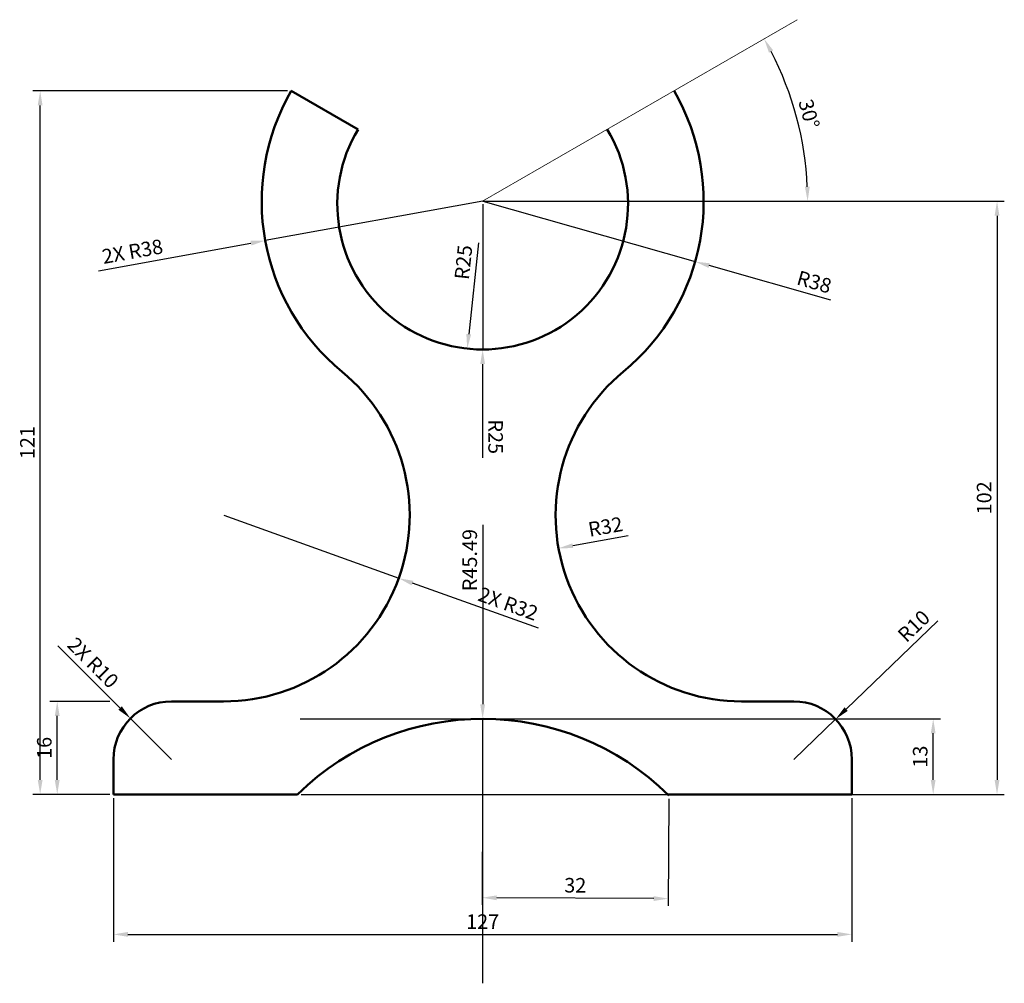
# Model space of a CAD drawing. Units: millimetres. Extents: x 195 to 364, y 6 to 172.
import ezdxf

# ---------------------------------------------------------------- set-up
doc = ezdxf.new("R2010")
doc.units = ezdxf.units.MM
for name, color, linetype, lineweight in [('M-CONS', 8, 'Continuous', 18), ('M-DIMS', 2, 'Continuous', 25), ('M-OUTL', 7, 'Continuous', 50)]:
    doc.layers.add(name, color=color, linetype=linetype, lineweight=lineweight)
doc.styles.get("Standard").update_dxf_attribs({"font": 'arial.ttf'})
doc.dimstyles.new('ISO-25', dxfattribs={"dimtxt": 2.5, "dimasz": 2.5, "dimexe": 1.25, "dimexo": 0.625, "dimtad": 1, "dimtxsty": 'Standard', "dimcen": 2.5, "dimadec": 0, "dimazin": 0, "dimtfac": 1, "dimtmove": 0, "dimatfit": 3, "dimfxl": 1, "dimarcsym": 0})

# ---------------------------------------------------------------- blocks, each defined once
blk = doc.blocks.new('*D1')
at = {"layer": 'Defpoints', "color": 0, "transparency": 16777216}
for p in [(328.48, 171.63), (329.42, 150.1), (274.38, 140.4), (274.38, 140.4), (329.43, 140.4)]:
    blk.add_point(p, dxfattribs=at)
at = {"layer": 'M-DIMS', "color": 0, "lineweight": -2, "transparency": 16777216}
blk.add_line((330.05, 140.4), (331.52, 140.4), dxfattribs=at)
blk.add_arc((274.38, 140.4), 55.89, 2.563, 27.437, dxfattribs=at)
at = {"layer": 'M-DIMS', "color": 0, "transparency": 16777216}
for points in [[(323.62, 165.95), (324.35, 166.35), (322.78, 168.34)], [(330.63, 142.91), (329.8, 142.89), (330.27, 140.4)]]:
    blk.add_solid(points, dxfattribs=at)
at = {"layer": 'M-DIMS', "color": 0, "transparency": 16777216, "insert": (330.2, 155.35), "char_height": 2.5, "attachment_point": 5, "rotation": 285}
blk.add_mtext('30°', dxfattribs=at)
blk = doc.blocks.new('*D2')
at = {"layer": 'Defpoints', "color": 0, "transparency": 16777216}
for p in [(274.38, 139.91), (271.72, 115.06)]:
    blk.add_point(p, dxfattribs=at)
at = {"layer": 'M-DIMS', "color": 0, "lineweight": -2, "transparency": 16777216}
blk.add_line((273.67, 133.27), (271.98, 117.54), dxfattribs=at)
at = {"layer": 'M-DIMS', "color": 0, "transparency": 16777216}
blk.add_solid([(271.57, 117.59), (272.4, 117.5), (271.72, 115.06)], dxfattribs=at)
at = {"layer": 'M-DIMS', "color": 0, "transparency": 16777216, "insert": (271.39, 129.87), "char_height": 2.5, "attachment_point": 5, "rotation": 83.8896}
blk.add_mtext('R25', dxfattribs=at)
blk = doc.blocks.new('*D3')
at = {"layer": 'Defpoints', "color": 0, "transparency": 16777216}
for p in [(318.92, 86.4), (287.43, 80.72)]:
    blk.add_point(p, dxfattribs=at)
at = {"layer": 'M-DIMS', "color": 0, "lineweight": -2, "transparency": 16777216}
blk.add_line((299.43, 82.89), (289.89, 81.17), dxfattribs=at)
at = {"layer": 'M-DIMS', "color": 0, "transparency": 16777216}
blk.add_solid([(289.81, 81.58), (289.96, 80.76), (287.43, 80.72)], dxfattribs=at)
at = {"layer": 'M-DIMS', "color": 0, "transparency": 16777216, "insert": (295.55, 84.12), "char_height": 2.5, "attachment_point": 5, "rotation": 10.2105}
blk.add_mtext('R32', dxfattribs=at)
blk = doc.blocks.new('*D4')
at = {"layer": 'Defpoints', "color": 0, "transparency": 16777216}
for p in [(335.08, 51.33), (327.88, 44.4)]:
    blk.add_point(p, dxfattribs=at)
at = {"layer": 'M-DIMS', "color": 0, "lineweight": -2, "transparency": 16777216}
for p, q in [((352.67, 68.25), (336.88, 53.06)), ((327.88, 44.4), (335.08, 51.33))]:
    blk.add_line(p, q, dxfattribs=at)
at = {"layer": 'M-DIMS', "color": 0, "transparency": 16777216}
blk.add_solid([(336.6, 53.36), (337.17, 52.76), (335.08, 51.33)], dxfattribs=at)
at = {"layer": 'M-DIMS', "color": 0, "transparency": 16777216, "insert": (348.75, 67.12), "char_height": 2.5, "attachment_point": 5, "rotation": 43.8985}
blk.add_mtext('R10', dxfattribs=at)
blk = doc.blocks.new('*D5')
at = {"layer": 'Defpoints', "color": 0, "transparency": 16777216}
for p in [(274.38, 38.4), (306.38, 38.24), (274.29, 20.63)]:
    blk.add_point(p, dxfattribs=at)
at = {"layer": 'M-DIMS', "color": 0, "lineweight": -2, "transparency": 16777216}
for p, q in [((274.37, 37.77), (274.28, 19.38)), ((306.37, 37.61), (306.28, 19.22)), ((303.79, 20.48), (276.79, 20.62))]:
    blk.add_line(p, q, dxfattribs=at)
at = {"layer": 'M-DIMS', "color": 0, "transparency": 16777216}
for points in [[(276.79, 21.03), (276.79, 20.2), (274.29, 20.63)], [(303.79, 20.9), (303.79, 20.07), (306.29, 20.47)]]:
    blk.add_solid(points, dxfattribs=at)
at = {"layer": 'M-DIMS', "color": 0, "transparency": 16777216, "insert": (290.3, 22.45), "char_height": 2.5, "attachment_point": 5, "rotation": 359.7141}
blk.add_mtext('32', dxfattribs=at)
blk = doc.blocks.new('*D6')
at = {"layer": 'Defpoints', "color": 0, "transparency": 16777216}
for p in [(210.88, 38.4), (337.88, 38.4), (337.88, 14.32)]:
    blk.add_point(p, dxfattribs=at)
at = {"layer": 'M-DIMS', "color": 0, "lineweight": -2, "transparency": 16777216}
for p, q in [((210.88, 37.77), (210.88, 13.07)), ((337.88, 37.77), (337.88, 13.07)), ((213.38, 14.32), (335.38, 14.32))]:
    blk.add_line(p, q, dxfattribs=at)
at = {"layer": 'M-DIMS', "color": 0, "transparency": 16777216}
for points in [[(213.38, 14.74), (213.38, 13.9), (210.88, 14.32)], [(335.38, 14.74), (335.38, 13.9), (337.88, 14.32)]]:
    blk.add_solid(points, dxfattribs=at)
at = {"layer": 'M-DIMS', "color": 0, "transparency": 16777216, "insert": (274.38, 16.2), "char_height": 2.5, "attachment_point": 5}
blk.add_mtext('127', dxfattribs=at)
blk = doc.blocks.new('*D7')
at = {"layer": 'Defpoints', "color": 0, "transparency": 16777216}
for p in [(242.38, 51.4), (351.86, 51.4), (242.54, 38.4)]:
    blk.add_point(p, dxfattribs=at)
at = {"layer": 'M-DIMS', "color": 0, "lineweight": -2, "transparency": 16777216}
for p, q in [((243, 51.4), (353.11, 51.4)), ((351.86, 40.9), (351.86, 48.9)), ((243.16, 38.4), (353.11, 38.4))]:
    blk.add_line(p, q, dxfattribs=at)
at = {"layer": 'M-DIMS', "color": 0, "transparency": 16777216}
for points in [[(351.44, 48.9), (352.27, 48.9), (351.86, 51.4)], [(351.44, 40.9), (352.27, 40.9), (351.86, 38.4)]]:
    blk.add_solid(points, dxfattribs=at)
at = {"layer": 'M-DIMS', "color": 0, "transparency": 16777216, "insert": (349.95, 44.9), "char_height": 2.5, "attachment_point": 5, "rotation": 90}
blk.add_mtext('13', dxfattribs=at)
blk = doc.blocks.new('*D8')
at = {"layer": 'Defpoints', "color": 0, "transparency": 16777216}
for p in [(201.21, 54.4), (210.88, 54.4), (210.88, 38.4)]:
    blk.add_point(p, dxfattribs=at)
at = {"layer": 'M-DIMS', "color": 0, "lineweight": -2, "transparency": 16777216}
for p, q in [((210.25, 54.4), (199.96, 54.4)), ((201.21, 40.9), (201.21, 51.9)), ((210.25, 38.4), (199.96, 38.4))]:
    blk.add_line(p, q, dxfattribs=at)
at = {"layer": 'M-DIMS', "color": 0, "transparency": 16777216}
for points in [[(200.79, 51.9), (201.63, 51.9), (201.21, 54.4)], [(200.79, 40.9), (201.63, 40.9), (201.21, 38.4)]]:
    blk.add_solid(points, dxfattribs=at)
at = {"layer": 'M-DIMS', "color": 0, "transparency": 16777216, "insert": (199.31, 46.4), "char_height": 2.5, "attachment_point": 5, "rotation": 90}
blk.add_mtext('16', dxfattribs=at)
blk = doc.blocks.new('*D9')
at = {"layer": 'Defpoints', "color": 0, "transparency": 16777216}
for p in [(274.38, 140.4), (310.93, 130.02)]:
    blk.add_point(p, dxfattribs=at)
at = {"layer": 'M-DIMS', "color": 0, "lineweight": -2, "transparency": 16777216}
for p, q in [((274.38, 140.4), (310.93, 130.02)), ((334.28, 123.4), (313.34, 129.34))]:
    blk.add_line(p, q, dxfattribs=at)
at = {"layer": 'M-DIMS', "color": 0, "transparency": 16777216}
blk.add_solid([(313.45, 129.74), (313.23, 128.94), (310.93, 130.02)], dxfattribs=at)
at = {"layer": 'M-DIMS', "color": 0, "transparency": 16777216, "insert": (331.32, 126.22), "char_height": 2.5, "attachment_point": 5, "rotation": 344.1606}
blk.add_mtext('R38', dxfattribs=at)
blk = doc.blocks.new('*D10')
at = {"layer": 'Defpoints', "color": 0, "transparency": 16777216}
for p in [(274.38, 140.4), (274.38, 38.4), (362.84, 38.4)]:
    blk.add_point(p, dxfattribs=at)
at = {"layer": 'M-DIMS', "color": 0, "lineweight": -2, "transparency": 16777216}
for p, q in [((275, 140.4), (364.09, 140.4)), ((362.84, 137.9), (362.84, 40.9)), ((275, 38.4), (364.09, 38.4))]:
    blk.add_line(p, q, dxfattribs=at)
at = {"layer": 'M-DIMS', "color": 0, "transparency": 16777216}
for points in [[(362.42, 137.9), (363.26, 137.9), (362.84, 140.4)], [(362.42, 40.9), (363.26, 40.9), (362.84, 38.4)]]:
    blk.add_solid(points, dxfattribs=at)
at = {"layer": 'M-DIMS', "color": 0, "transparency": 16777216, "insert": (360.94, 89.4), "char_height": 2.5, "attachment_point": 5, "rotation": 90}
blk.add_mtext('102', dxfattribs=at)
blk = doc.blocks.new('*D11')
at = {"layer": 'Defpoints', "color": 0, "transparency": 16777216}
for p in [(198.28, 159.4), (241.47, 159.4), (210.88, 38.4)]:
    blk.add_point(p, dxfattribs=at)
at = {"layer": 'M-DIMS', "color": 0, "lineweight": -2, "transparency": 16777216}
for p, q in [((240.84, 159.4), (197.03, 159.4)), ((198.28, 40.9), (198.28, 156.9)), ((210.25, 38.4), (197.03, 38.4))]:
    blk.add_line(p, q, dxfattribs=at)
at = {"layer": 'M-DIMS', "color": 0, "transparency": 16777216}
for points in [[(197.86, 156.9), (198.69, 156.9), (198.28, 159.4)], [(197.86, 40.9), (198.69, 40.9), (198.28, 38.4)]]:
    blk.add_solid(points, dxfattribs=at)
at = {"layer": 'M-DIMS', "color": 0, "transparency": 16777216, "insert": (196.4, 98.9), "char_height": 2.5, "attachment_point": 5, "rotation": 90}
blk.add_mtext('121', dxfattribs=at)
blk = doc.blocks.new('*D12')
at = {"layer": 'Defpoints', "color": 0, "transparency": 16777216}
for p in [(274.38, 140.4), (236.98, 133.64)]:
    blk.add_point(p, dxfattribs=at)
at = {"layer": 'M-DIMS', "color": 0, "lineweight": -2, "transparency": 16777216}
for p, q in [((274.38, 140.4), (236.98, 133.64)), ((208.33, 128.46), (234.52, 133.2))]:
    blk.add_line(p, q, dxfattribs=at)
at = {"layer": 'M-DIMS', "color": 0, "transparency": 16777216}
blk.add_solid([(234.45, 133.61), (234.6, 132.79), (236.98, 133.64)], dxfattribs=at)
at = {"layer": 'M-DIMS', "color": 0, "transparency": 16777216, "insert": (214.21, 131.46), "char_height": 2.5, "attachment_point": 5, "rotation": 10.2416}
blk.add_mtext('2X R38', dxfattribs=at)
blk = doc.blocks.new('*D13')
at = {"layer": 'Defpoints', "color": 0, "transparency": 16777216}
for p in [(229.84, 86.4), (259.95, 75.58)]:
    blk.add_point(p, dxfattribs=at)
at = {"layer": 'M-DIMS', "color": 0, "lineweight": -2, "transparency": 16777216}
for p, q in [((229.84, 86.4), (259.95, 75.58)), ((283.96, 66.96), (262.3, 74.73))]:
    blk.add_line(p, q, dxfattribs=at)
at = {"layer": 'M-DIMS', "color": 0, "transparency": 16777216}
blk.add_solid([(262.45, 75.13), (262.16, 74.34), (259.95, 75.58)], dxfattribs=at)
at = {"layer": 'M-DIMS', "color": 0, "transparency": 16777216, "insert": (278.66, 70.88), "char_height": 2.5, "attachment_point": 5, "rotation": 340.2407}
blk.add_mtext('2X R32', dxfattribs=at)
blk = doc.blocks.new('*D14')
at = {"layer": 'Defpoints', "color": 0, "transparency": 16777216}
for p in [(274.38, 139.91), (274.38, 114.91)]:
    blk.add_point(p, dxfattribs=at)
at = {"layer": 'M-DIMS', "color": 0, "lineweight": -2, "transparency": 16777216}
for p, q in [((274.38, 139.91), (274.38, 114.91)), ((274.38, 96.29), (274.38, 112.41))]:
    blk.add_line(p, q, dxfattribs=at)
at = {"layer": 'M-DIMS', "color": 0, "transparency": 16777216}
blk.add_solid([(274.79, 112.41), (273.96, 112.41), (274.38, 114.91)], dxfattribs=at)
at = {"layer": 'M-DIMS', "color": 0, "transparency": 16777216, "insert": (276.28, 99.91), "char_height": 2.5, "attachment_point": 5, "rotation": 270.0005}
blk.add_mtext('R25', dxfattribs=at)
blk = doc.blocks.new('*D15')
at = {"layer": 'Defpoints', "color": 0, "transparency": 16777216}
for p in [(213.81, 51.47), (220.88, 44.4)]:
    blk.add_point(p, dxfattribs=at)
at = {"layer": 'M-DIMS', "color": 0, "lineweight": -2, "transparency": 16777216}
for p, q in [((201.34, 63.93), (212.04, 53.24)), ((220.88, 44.4), (213.81, 51.47))]:
    blk.add_line(p, q, dxfattribs=at)
at = {"layer": 'M-DIMS', "color": 0, "transparency": 16777216}
blk.add_solid([(212.33, 53.53), (211.74, 52.94), (213.81, 51.47)], dxfattribs=at)
at = {"layer": 'M-DIMS', "color": 0, "transparency": 16777216, "insert": (207.15, 60.81), "char_height": 2.5, "attachment_point": 5, "rotation": 315.0006}
blk.add_mtext('2X R10', dxfattribs=at)
blk = doc.blocks.new('*D16')
at = {"layer": 'Defpoints', "color": 0, "transparency": 16777216}
for p in [(274.38, 51.4), (274.38, 5.91)]:
    blk.add_point(p, dxfattribs=at)
at = {"layer": 'M-DIMS', "color": 0, "lineweight": -2, "transparency": 16777216}
for p, q in [((274.38, 84.73), (274.38, 53.9)), ((274.38, 5.91), (274.38, 51.4))]:
    blk.add_line(p, q, dxfattribs=at)
at = {"layer": 'M-DIMS', "color": 0, "transparency": 16777216}
blk.add_solid([(273.96, 53.9), (274.79, 53.9), (274.38, 51.4)], dxfattribs=at)
at = {"layer": 'M-DIMS', "color": 0, "transparency": 16777216, "insert": (272.48, 78.69), "char_height": 2.5, "attachment_point": 5, "rotation": 89.9997}
blk.add_mtext('R45.49', dxfattribs=at)

msp = doc.modelspace()

# ---------------------------------------------------------------- linework, layer by layer
at = {"layer": 'M-CONS'}
for q in [(328.476, 171.63), (329.426, 140.396)]:
    msp.add_line((274.378, 140.396), q, dxfattribs=at)
at = {"layer": 'M-OUTL'}
for p, q in [((252.939, 152.774), (241.469, 159.396)), ((229.836, 54.396), (220.878, 54.396)), ((327.878, 54.396), (318.92, 54.396)), ((210.878, 38.396), (210.878, 44.396)), ((337.878, 38.396), (337.878, 44.396)), ((210.878, 38.396), (242.54, 38.396)), ((210.878, 38.396), (242.54, 38.396)), ((242.54, 38.396), (242.378, 38.396)), ((306.216, 38.396), (306.378, 38.396)), ((306.216, 38.396), (337.878, 38.396)), ((306.378, 38.396), (306.378, 38.237))]:
    msp.add_line(p, q, dxfattribs=at)
for centre, radius, start, end in [((274.378, 140.396), 38, 150, 230.48235), ((274.378, 140.396), 38, 309.51765, 30), ((274.378, 139.914), 25, 149.04169, 30.95831), ((229.836, 86.396), 32, 270, 50.48235), ((318.92, 86.396), 32, 129.51765, 270), ((220.878, 44.396), 10, 90, 180), ((327.878, 44.396), 10, 0, 90), ((274.378, 5.91), 45.487, 45.29113, 134.42223)]:
    msp.add_arc(centre, radius, start, end, dxfattribs=at)

# ---------------------------------------------------------------- dimensions: what is measured, and where the dimension line sits
at = {"layer": 'M-DIMS'}
dim = msp.add_angular_dim_2l(base=(329.422, 150.102), line1=((274.378, 140.396), (328.476, 171.63)), line2=((274.378, 140.396), (329.426, 140.396)), dimstyle='ISO-25', override={"dimclrd": 0, "dimclre": 0, "dimclrt": 0}, dxfattribs=at)
dim.commit()
dim.dimension.update_dxf_attribs({"geometry": '*D1', "text_midpoint": (330.204, 155.355)})
for base, p1, p2, override, picture, middle in [((198.278, 159.396), (210.878, 38.396), (241.469, 159.396), {"dimdec": 0, "dimlfac": 1, "dimrnd": 0, "dimzin": 0, "dimdsep": 46, "dimlunit": 2}, '*D11', (196.398, 98.896)), ((362.84, 38.396), (274.378, 140.396), (274.378, 38.396), {"dimclrd": 0, "dimclre": 0, "dimclrt": 0}, '*D10', (360.939, 89.396)), ((201.211, 54.396), (210.878, 38.396), (210.878, 54.396), {"dimclrd": 0, "dimclre": 0, "dimclrt": 0}, '*D8', (199.31, 46.396)), ((351.856, 51.396), (242.54, 38.396), (242.378, 51.396), {"dimclrd": 0, "dimclre": 0, "dimclrt": 0}, '*D7', (349.954, 44.896))]:
    dim = msp.add_linear_dim(base=base, p1=p1, p2=p2, angle=90, dimstyle='ISO-25', override=override, dxfattribs=at)
    dim.commit()
    dim.dimension.update_dxf_attribs({"geometry": picture, "text_midpoint": middle})
for center, mpoint, picture, middle in [((274.378, 140.396), (236.983, 133.64), '*D12', (214.547, 129.586)), ((229.836, 86.396), (259.952, 75.578), '*D13', (278.021, 69.087))]:
    dim = msp.add_radius_dim(center=center, mpoint=mpoint, text='2X <>', dimstyle='ISO-25', override={"dimdec": 0, "dimlfac": 1, "dimrnd": 0, "dimzin": 0, "dimdsep": 46, "dimlunit": 2}, dxfattribs=at)
    dim.commit()
    dim.dimension.update_dxf_attribs({"geometry": picture, "text_midpoint": middle, "dimtype": 164})
for center, mpoint, override, picture, middle in [((274.378, 139.914), (271.717, 115.056), {"dimclrd": 0, "dimclre": 0, "dimclrt": 0}, '*D2', (273.281, 129.672)), ((274.378, 139.914), (274.378, 114.914), {"dimdec": 0, "dimlfac": 1, "dimrnd": 0, "dimzin": 0, "dimdsep": 46, "dimlunit": 2}, '*D14', (274.378, 99.914)), ((274.378, 140.396), (310.935, 130.025), {"dimclrd": 0, "dimclre": 0, "dimclrt": 0}, '*D9', (330.804, 124.387)), ((318.92, 86.396), (287.427, 80.724), {"dimclrd": 0, "dimclre": 0, "dimclrt": 0}, '*D3', (295.89, 82.248)), ((274.378, 5.91), (274.378, 51.396), {"dimdec": 2, "dimlfac": 1, "dimrnd": 0, "dimzin": 0, "dimdsep": 46, "dimlunit": 2}, '*D16', (274.378, 78.688)), ((327.878, 44.396), (335.083, 51.33), {"dimclrd": 0, "dimclre": 0, "dimclrt": 0}, '*D4', (350.072, 65.753))]:
    dim = msp.add_radius_dim(center=center, mpoint=mpoint, dimstyle='ISO-25', override=override, dxfattribs=at)
    dim.commit()
    dim.dimension.update_dxf_attribs({"geometry": picture, "text_midpoint": middle, "dimtype": 164})
dim = msp.add_radius_dim(center=(220.878, 44.396), mpoint=(213.807, 51.467), text='2X <>', dimstyle='ISO-25', override={"dimdec": 0, "dimlfac": 1, "dimrnd": 0, "dimzin": 0, "dimdsep": 46, "dimlunit": 2}, dxfattribs=at)
dim.commit()
dim.dimension.update_dxf_attribs({"geometry": '*D15', "text_midpoint": (207.15, 60.813)})
dim = msp.add_linear_dim(base=(337.878, 14.32), p1=(210.878, 38.396), p2=(337.878, 38.396), dimstyle='ISO-25', override={"dimclrd": 0, "dimclre": 0, "dimclrt": 0}, dxfattribs=at)
dim.commit()
dim.dimension.update_dxf_attribs({"geometry": '*D6', "text_midpoint": (274.378, 16.2)})
dim = msp.add_aligned_dim(p1=(306.378, 38.237), p2=(274.378, 38.396), distance=17.767, dimstyle='ISO-25', override={"dimclrd": 0, "dimclre": 0, "dimclrt": 0}, dxfattribs=at)
dim.commit()
dim.dimension.update_dxf_attribs({"geometry": '*D5', "text_midpoint": (290.299, 22.452)})

doc.saveas('drawing.dxf')
